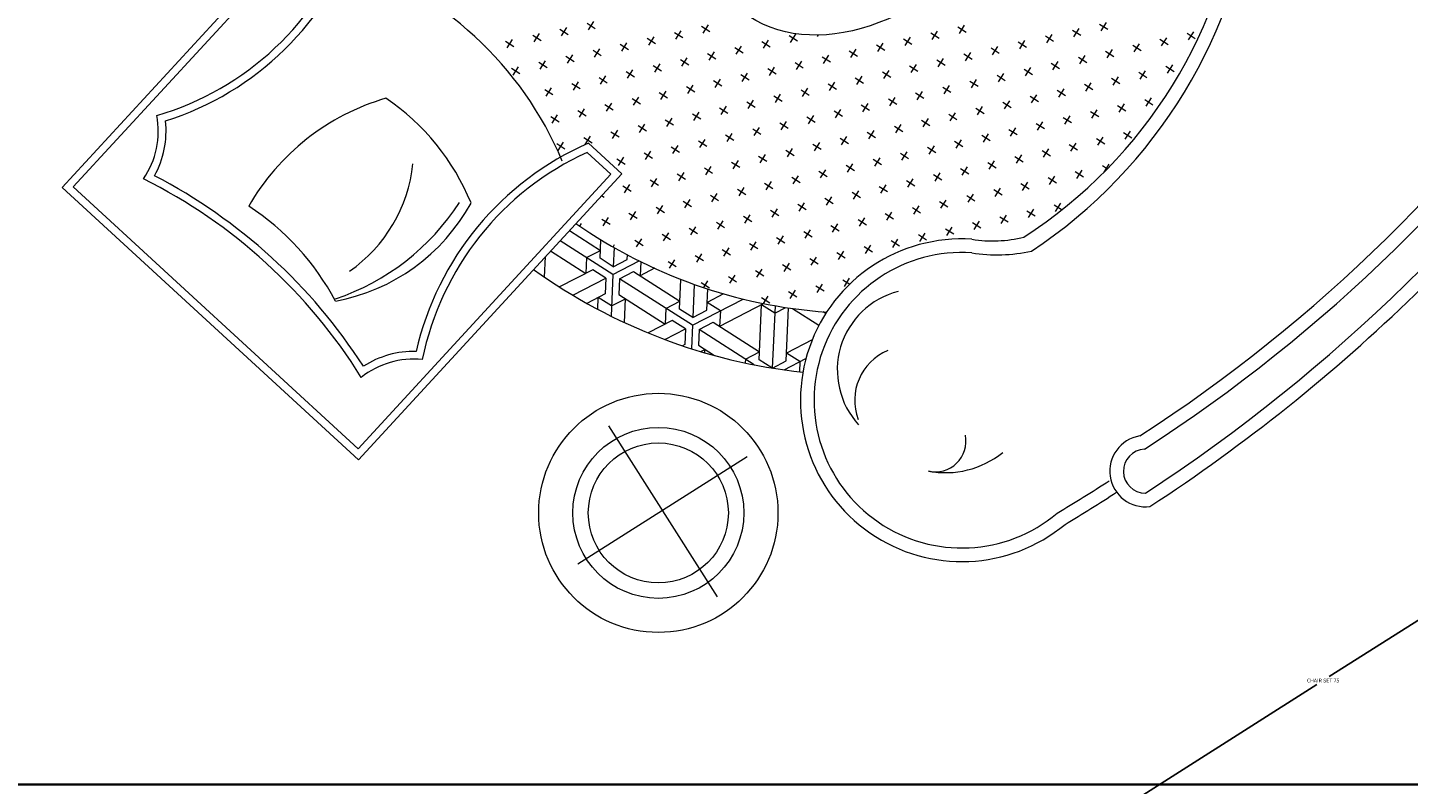
# Model space of a CAD drawing. Units: inches. Extents: x -4843 to -3402, y -164 to 3629.
# Tile 10 of 22: x -4532 to -4467, y 828 to 864. Entities that reach past the tile are written whole.
import ezdxf

# ---------------------------------------------------------------- set-up
doc = ezdxf.new("R2010")
doc.units = ezdxf.units.IN
for name, color, linetype, lineweight in [('A-ANNO-DIMS', 2, 'Continuous', 18), ('furniture', 6, 'Continuous', 18), ('walls', 7, 'Continuous', 35)]:
    doc.layers.add(name, color=color, linetype=linetype, lineweight=lineweight)
doc.styles.get("Standard").update_dxf_attribs({"font": 'arial.ttf'})
doc.dimstyles.get("Standard").update_dxf_attribs({"dimtxt": 0.18, "dimasz": 0.18, "dimexe": 0.18, "dimexo": 0.0625, "dimgap": 0.09, "dimtad": 0, "dimtih": 1, "dimtoh": 1, "dimdec": 4, "dimzin": 0, "dimdsep": 46, "dimtxsty": 'Standard', "dimcen": 0.09, "dimadec": 0, "dimazin": 0, "dimtfac": 1, "dimtdec": 4, "dimtofl": 0, "dimtmove": 0, "dimatfit": 3, "dimfxl": 1, "dimtolj": 1, "dimtzin": 0, "dimarcsym": 0})

# ---------------------------------------------------------------- blocks, each defined once
blk = doc.blocks.new('A$C30AE1D3B')
for p, q in [((2417.8, 2221.8, -685.7), (2417.8, 1828.4, -685.7)), ((2611.9, 2022.7, -685.7), (2223.7, 2022.7, -685.7)), ((1343.9, 1928.3, -685.7), (1327.1, 1920.4, -685.7)), ((1464.1, 1942.3, -685.7), (1446.8, 1934.2, -685.7)), ((1459.4, 1929.6, -685.7), (1451.7, 1946.1, -685.7)), ((1510.1, 1911.2, -685.7), (1502, 1928.4, -685.7)), ((2038.5, 1922.1, -685.7), (2049.7, 1938.2, -685.7)), ((1270.7, 1883.6, -685.7), (1262.6, 1900.9, -685.7)), ((1339.8, 1915.8, -685.7), (1334.9, 1926.2, -685.7)), ((1395, 1910.1, -685.7), (1377.7, 1902, -685.7)), ((1390.4, 1897.4, -685.7), (1382.3, 1914.7, -685.7)), ((1514.7, 1923.8, -685.7), (1497.4, 1915.8, -685.7)), ((1565.3, 1905.4, -685.7), (1548.1, 1897.3, -685.7)), ((1560.7, 1892.7, -685.7), (1552.7, 1910, -685.7)), ((2060.1, 1907, -685.7), (2001, 1822.6, -685.7)), ((2020.9, 1804.9, -685.7), (2090.2, 1904, -685.7)), ((2072.8, 1919.1, -685.7), (2025.3, 1923.3, -685.7)), ((2038.5, 1922.1, -685.7), (2051.4, 1894.5, -685.7)), ((2089.7, 1904.4, -685.7), (2060.1, 1907, -685.7)), ((2091, 1903.3, -685.7), (2103.3, 1876.7, -685.7)), ((1275.3, 1896.3, -685.7), (1258, 1888.2, -685.7)), ((1325.9, 1877.8, -685.7), (1308.7, 1869.8, -685.7)), ((1321.3, 1865.2, -685.7), (1313.3, 1882.5, -685.7)), ((1445.6, 1891.6, -685.7), (1428.4, 1883.6, -685.7)), ((1441, 1879, -685.7), (1433, 1896.2, -685.7)), ((1491.7, 1860.5, -685.7), (1483.6, 1877.8, -685.7)), ((1616, 1887, -685.7), (1598.7, 1878.9, -685.7)), ((1611.3, 1874.3, -685.7), (1603.3, 1891.6, -685.7)), ((1995.2, 1827.5, -685.7), (1969.6, 1882.5, -685.7)), ((1995.9, 1899.4, -685.7), (2051.4, 1894.5, -685.7)), ((2103.4, 1876.7, -685.7), (2042.2, 1789.3, -685.7)), ((2116.4, 1879.9, -685.7), (2170.1, 1764.9, -685.7)), ((1206.2, 1864.1, -685.7), (1189, 1856, -685.7)), ((1201.6, 1851.4, -685.7), (1193.6, 1868.7, -685.7)), ((1252.3, 1833, -685.7), (1244.2, 1850.3, -685.7)), ((1376.6, 1859.4, -685.7), (1359.3, 1851.4, -685.7)), ((1372, 1846.8, -685.7), (1363.9, 1864, -685.7)), ((1496.3, 1873.2, -685.7), (1479, 1865.1, -685.7)), ((1546.9, 1854.8, -685.7), (1529.6, 1846.7, -685.7)), ((1542.3, 1842.1, -685.7), (1534.2, 1859.4, -685.7)), ((1666.6, 1868.5, -685.7), (1649.3, 1860.5, -685.7)), ((1662, 1855.9, -685.7), (1653.9, 1873.1, -685.7)), ((1717.2, 1850.1, -685.7), (1700, 1842.1, -685.7)), ((1712.6, 1837.5, -685.7), (1704.6, 1854.7, -685.7)), ((1882.9, 1832.8, -685.7), (1876.2, 1847.2, -685.7)), ((1946.2, 1870.3, -685.7), (1948.8, 1864.7, -685.7)), ((2139.7, 1767.6, -685.7), (2094.6, 1864.2, -685.7)), ((2125, 1861.6, -685.7), (2094.6, 1864.2, -685.7)), ((2125, 1861.6, -685.7), (2129.2, 1867.6, -685.7)), ((1137.2, 1831.9, -685.7), (1119.9, 1823.8, -685.7)), ((1132.6, 1819.2, -685.7), (1124.5, 1836.5, -685.7)), ((1256.9, 1845.6, -685.7), (1239.6, 1837.6, -685.7)), ((1307.5, 1827.2, -685.7), (1290.2, 1819.2, -685.7)), ((1302.9, 1814.6, -685.7), (1294.8, 1831.8, -685.7)), ((1427.2, 1841, -685.7), (1409.9, 1832.9, -685.7)), ((1422.6, 1828.3, -685.7), (1414.5, 1845.6, -685.7)), ((1477.8, 1822.6, -685.7), (1460.6, 1814.5, -685.7)), ((1473.2, 1809.9, -685.7), (1465.2, 1827.2, -685.7)), ((1597.5, 1836.3, -685.7), (1580.3, 1828.3, -685.7)), ((1592.9, 1823.7, -685.7), (1584.9, 1840.9, -685.7)), ((1643.5, 1805.3, -685.7), (1635.5, 1822.5, -685.7)), ((1767.8, 1831.7, -685.7), (1750.6, 1823.6, -685.7)), ((1763.2, 1819, -685.7), (1755.2, 1836.3, -685.7)), ((1887.5, 1845.5, -685.7), (1870.3, 1837.4, -685.7)), ((1938.2, 1827, -685.7), (1920.9, 1819, -685.7)), ((1933.6, 1814.4, -685.7), (1925.5, 1831.6, -685.7)), ((2187.5, 1789.9, -685.7), (2172, 1823.3, -685.7)), ((1068.1, 1799.7, -685.7), (1050.9, 1791.6, -685.7)), ((1063.5, 1787, -685.7), (1055.5, 1804.3, -685.7)), ((1187.8, 1813.4, -685.7), (1170.5, 1805.4, -685.7)), ((1183.2, 1800.8, -685.7), (1175.2, 1818, -685.7)), ((1238.4, 1795, -685.7), (1221.2, 1787, -685.7)), ((1233.8, 1782.4, -685.7), (1225.8, 1799.6, -685.7)), ((1358.1, 1808.8, -685.7), (1340.9, 1800.7, -685.7)), ((1353.5, 1796.1, -685.7), (1345.5, 1813.4, -685.7)), ((1404.2, 1777.7, -685.7), (1396.1, 1795, -685.7)), ((1528.5, 1804.1, -685.7), (1511.2, 1796.1, -685.7)), ((1523.9, 1791.5, -685.7), (1515.8, 1808.7, -685.7)), ((1648.2, 1817.9, -685.7), (1630.9, 1809.9, -685.7)), ((1698.8, 1799.5, -685.7), (1681.5, 1791.4, -685.7)), ((1694.2, 1786.8, -685.7), (1686.1, 1804.1, -685.7)), ((1818.5, 1813.3, -685.7), (1801.2, 1805.2, -685.7)), ((1813.9, 1800.6, -685.7), (1805.8, 1817.9, -685.7)), ((1869.1, 1794.8, -685.7), (1851.8, 1786.8, -685.7)), ((1864.5, 1782.2, -685.7), (1856.5, 1799.4, -685.7)), ((1988.8, 1808.6, -685.7), (1971.5, 1800.6, -685.7)), ((1984.2, 1795.9, -685.7), (1976.1, 1813.2, -685.7)), ((2029.3, 1816.9, -685.7), (2005, 1819.1, -685.7)), ((2034.8, 1777.5, -685.7), (2026.8, 1794.8, -685.7)), ((2029.3, 1817, -685.7), (2042.2, 1789.3, -685.7)), ((2184.8, 1808.9, -685.7), (2181.1, 1803.7, -685.7)), ((2190.1, 1802.9, -685.7), (2181.1, 1803.7, -685.7)), ((1118.8, 1781.2, -685.7), (1101.5, 1773.2, -685.7)), ((1114.1, 1768.6, -685.7), (1106.1, 1785.8, -685.7)), ((1164.8, 1750.2, -685.7), (1156.7, 1767.4, -685.7)), ((1289.1, 1776.6, -685.7), (1271.8, 1768.5, -685.7)), ((1284.5, 1763.9, -685.7), (1276.4, 1781.2, -685.7)), ((1408.8, 1790.4, -685.7), (1391.5, 1782.3, -685.7)), ((1459.4, 1771.9, -685.7), (1442.1, 1763.9, -685.7)), ((1454.8, 1759.3, -685.7), (1446.7, 1776.5, -685.7)), ((1579.1, 1785.7, -685.7), (1561.8, 1777.7, -685.7)), ((1574.5, 1773, -685.7), (1566.4, 1790.3, -685.7)), ((1629.7, 1767.3, -685.7), (1612.5, 1759.2, -685.7)), ((1625.1, 1754.6, -685.7), (1617.1, 1771.9, -685.7)), ((1749.4, 1781.1, -685.7), (1732.2, 1773, -685.7)), ((1744.8, 1768.4, -685.7), (1736.8, 1785.7, -685.7)), ((1795.4, 1750, -685.7), (1787.4, 1767.2, -685.7)), ((1919.7, 1776.4, -685.7), (1902.5, 1768.3, -685.7)), ((1915.1, 1763.7, -685.7), (1907.1, 1781, -685.7)), ((2037.6, 1789.3, -685.7), (2022.2, 1782.1, -685.7)), ((2037.1, 1789.8, -685.7), (2133.3, 1781.4, -685.7)), ((2115.8, 1756.4, -685.7), (2133.3, 1781.4, -685.7)), ((2170.1, 1764.9, -685.7), (2139.7, 1767.5, -685.7)), ((2170.1, 1764.9, -685.7), (2187.6, 1789.9, -685.7)), ((2176.5, 1751.1, -685.7), (2202.5, 1788.2, -685.7)), ((2191.7, 1749.8, -685.7), (2209.2, 1774.7, -685.7)), ((2209.2, 1774.7, -685.7), (2214, 1774.3, -685.7)), ((1169.4, 1762.8, -685.7), (1152.1, 1754.8, -685.7)), ((1220, 1744.4, -685.7), (1202.8, 1736.3, -685.7)), ((1215.4, 1731.7, -685.7), (1207.4, 1749, -685.7)), ((1339.7, 1758.2, -685.7), (1322.4, 1750.1, -685.7)), ((1335.1, 1745.5, -685.7), (1327.1, 1762.8, -685.7)), ((1390.3, 1739.7, -685.7), (1373.1, 1731.7, -685.7)), ((1385.7, 1727.1, -685.7), (1377.7, 1744.3, -685.7)), ((1510, 1753.5, -685.7), (1492.8, 1745.5, -685.7)), ((1505.4, 1740.8, -685.7), (1497.4, 1758.1, -685.7)), ((1556.1, 1722.4, -685.7), (1548, 1739.7, -685.7)), ((1680.4, 1748.8, -685.7), (1663.1, 1740.8, -685.7)), ((1675.8, 1736.2, -685.7), (1667.7, 1753.5, -685.7)), ((1800.1, 1762.6, -685.7), (1782.8, 1754.6, -685.7)), ((1850.7, 1744.2, -685.7), (1833.4, 1736.1, -685.7)), ((1846.1, 1731.5, -685.7), (1838, 1748.8, -685.7)), ((1970.4, 1758, -685.7), (1953.1, 1749.9, -685.7)), ((1965.8, 1745.3, -685.7), (1957.7, 1762.6, -685.7)), ((2016.4, 1726.9, -685.7), (2008.4, 1744.1, -685.7)), ((2176.5, 1751.1, -685.7), (2066.2, 1760.7, -685.7)), ((2137.4, 1741.3, -685.7), (2113.7, 1707.4, -685.7)), ((2115.8, 1756.4, -685.7), (2128.6, 1728.8, -685.7)), ((2167.8, 1738.6, -685.7), (2137.4, 1741.2, -685.7)), ((2176.5, 1751.1, -685.7), (2247.3, 1599.2, -685.7)), ((2191.7, 1749.8, -685.7), (2204.6, 1722.1, -685.7)), ((2236.2, 1745.8, -685.7), (2191.7, 1749.7, -685.7)), ((1270.6, 1726, -685.7), (1253.4, 1717.9, -685.7)), ((1266, 1713.3, -685.7), (1258, 1730.6, -685.7)), ((1441, 1721.3, -685.7), (1423.7, 1713.2, -685.7)), ((1436.4, 1708.6, -685.7), (1428.3, 1725.9, -685.7)), ((1560.7, 1735.1, -685.7), (1543.4, 1727, -685.7)), ((1611.3, 1716.6, -685.7), (1594, 1708.6, -685.7)), ((1606.7, 1704, -685.7), (1598.6, 1721.3, -685.7)), ((1731, 1730.4, -685.7), (1713.7, 1722.4, -685.7)), ((1726.4, 1717.8, -685.7), (1718.3, 1735, -685.7)), ((1777, 1699.3, -685.7), (1769, 1716.6, -685.7)), ((1901.3, 1725.8, -685.7), (1884.1, 1717.7, -685.7)), ((1896.7, 1713.1, -685.7), (1888.7, 1730.4, -685.7)), ((2021, 1739.5, -685.7), (2003.7, 1731.5, -685.7)), ((2071.6, 1721.1, -685.7), (2054.4, 1713.1, -685.7)), ((2067, 1708.5, -685.7), (2059, 1725.7, -685.7)), ((2092.7, 1731.9, -685.7), (2128.7, 1728.8, -685.7)), ((2130.9, 1686, -685.7), (2167.8, 1738.6, -685.7)), ((2167.8, 1738.6, -685.7), (2180.6, 1711, -685.7)), ((2202.3, 1695.8, -685.7), (2219.8, 1720.8, -685.7)), ((2204.6, 1722.1, -685.7), (2256.9, 1717.5, -685.7)), ((2264.8, 1624.1, -685.7), (2219.7, 1720.8, -685.7)), ((1201.6, 1693.7, -685.7), (1184.3, 1685.7, -685.7)), ((1197, 1681.1, -685.7), (1188.9, 1698.4, -685.7)), ((1321.3, 1707.5, -685.7), (1304, 1699.5, -685.7)), ((1316.7, 1694.9, -685.7), (1308.6, 1712.1, -685.7)), ((1371.9, 1689.1, -685.7), (1354.6, 1681, -685.7)), ((1367.3, 1676.4, -685.7), (1359.3, 1693.7, -685.7)), ((1491.6, 1702.9, -685.7), (1474.3, 1694.8, -685.7)), ((1487, 1690.2, -685.7), (1478.9, 1707.5, -685.7)), ((1537.6, 1671.8, -685.7), (1529.6, 1689, -685.7)), ((1661.9, 1698.2, -685.7), (1644.7, 1690.2, -685.7)), ((1657.3, 1685.6, -685.7), (1649.3, 1702.8, -685.7)), ((1781.6, 1712, -685.7), (1764.4, 1703.9, -685.7)), ((1832.3, 1693.6, -685.7), (1815, 1685.5, -685.7)), ((1827.6, 1680.9, -685.7), (1819.6, 1698.2, -685.7)), ((1951.9, 1707.3, -685.7), (1934.7, 1699.3, -685.7)), ((1947.3, 1694.7, -685.7), (1939.3, 1711.9, -685.7)), ((2002.6, 1688.9, -685.7), (1985.3, 1680.9, -685.7)), ((1998, 1676.3, -685.7), (1989.9, 1693.5, -685.7)), ((2118.9, 1701.1, -685.7), (2105, 1694.6, -685.7)), ((2117.7, 1690, -685.7), (2109.6, 1707.3, -685.7)), ((2180.7, 1711, -685.7), (2147.7, 1663.9, -685.7)), ((2217, 1601.8, -685.7), (2171.9, 1698.5, -685.7)), ((2202.3, 1695.8, -685.7), (2171.9, 1698.5, -685.7)), ((1252.2, 1675.3, -685.7), (1235, 1667.3, -685.7)), ((1247.6, 1662.7, -685.7), (1239.6, 1679.9, -685.7)), ((1298.2, 1644.2, -685.7), (1290.2, 1661.5, -685.7)), ((1422.5, 1670.7, -685.7), (1405.3, 1662.6, -685.7)), ((1417.9, 1658, -685.7), (1409.9, 1675.3, -685.7)), ((1542.2, 1684.4, -685.7), (1525, 1676.4, -685.7)), ((1592.9, 1666, -685.7), (1575.6, 1658, -685.7)), ((1588.3, 1653.4, -685.7), (1580.2, 1670.6, -685.7)), ((1712.6, 1679.8, -685.7), (1695.3, 1671.7, -685.7)), ((1708, 1667.1, -685.7), (1699.9, 1684.4, -685.7)), ((1763.2, 1661.4, -685.7), (1745.9, 1653.3, -685.7)), ((1758.6, 1648.7, -685.7), (1750.5, 1666, -685.7)), ((1882.9, 1675.1, -685.7), (1865.6, 1667.1, -685.7)), ((1878.3, 1662.5, -685.7), (1870.2, 1679.7, -685.7)), ((1928.9, 1644, -685.7), (1920.9, 1661.3, -685.7)), ((2053.2, 1670.5, -685.7), (2035.9, 1662.4, -685.7)), ((2048.6, 1657.8, -685.7), (2040.6, 1675.1, -685.7)), ((2284.9, 1675.8, -685.7), (2258.4, 1637.9, -685.7)), ((1302.9, 1656.9, -685.7), (1285.6, 1648.8, -685.7)), ((1353.5, 1638.5, -685.7), (1336.2, 1630.4, -685.7)), ((1348.9, 1625.8, -685.7), (1340.8, 1643.1, -685.7)), ((1473.2, 1652.2, -685.7), (1455.9, 1644.2, -685.7)), ((1468.6, 1639.6, -685.7), (1460.5, 1656.8, -685.7)), ((1523.8, 1633.8, -685.7), (1506.5, 1625.8, -685.7)), ((1519.2, 1621.2, -685.7), (1511.2, 1638.4, -685.7)), ((1643.5, 1647.6, -685.7), (1626.2, 1639.5, -685.7)), ((1638.9, 1634.9, -685.7), (1630.8, 1652.2, -685.7)), ((1689.5, 1616.5, -685.7), (1681.5, 1633.8, -685.7)), ((1813.8, 1642.9, -685.7), (1796.6, 1634.9, -685.7)), ((1809.2, 1630.3, -685.7), (1801.2, 1647.5, -685.7)), ((1933.5, 1656.7, -685.7), (1916.3, 1648.7, -685.7)), ((1984.2, 1638.3, -685.7), (1966.9, 1630.2, -685.7)), ((1979.5, 1625.6, -685.7), (1971.5, 1642.9, -685.7)), ((2103.8, 1652.1, -685.7), (2086.6, 1644, -685.7)), ((2099.2, 1639.4, -685.7), (2091.2, 1656.7, -685.7)), ((2154.5, 1633.6, -685.7), (2137.2, 1625.6, -685.7)), ((2149.9, 1621, -685.7), (2141.8, 1638.2, -685.7)), ((2253.8, 1585.3, -685.7), (2300.1, 1651.4, -685.7)), ((2288.8, 1635.3, -685.7), (2258.4, 1637.9, -685.7)), ((2288.7, 1635.3, -685.7), (2301.6, 1607.7, -685.7)), ((1404.1, 1620, -685.7), (1386.9, 1612, -685.7)), ((1399.5, 1607.4, -685.7), (1391.5, 1624.6, -685.7)), ((1450.1, 1588.9, -685.7), (1442.1, 1606.2, -685.7)), ((1574.4, 1615.4, -685.7), (1557.2, 1607.3, -685.7)), ((1569.8, 1602.7, -685.7), (1561.8, 1620, -685.7)), ((1694.1, 1629.2, -685.7), (1676.9, 1621.1, -685.7)), ((1744.8, 1610.7, -685.7), (1727.5, 1602.7, -685.7)), ((1740.2, 1598.1, -685.7), (1732.1, 1615.3, -685.7)), ((1864.5, 1624.5, -685.7), (1847.2, 1616.5, -685.7)), ((1859.9, 1611.8, -685.7), (1851.8, 1629.1, -685.7)), ((1915.1, 1606.1, -685.7), (1897.8, 1598, -685.7)), ((1910.5, 1593.4, -685.7), (1902.4, 1610.7, -685.7)), ((2034.8, 1619.8, -685.7), (2017.5, 1611.8, -685.7)), ((2030.2, 1607.2, -685.7), (2022.1, 1624.5, -685.7)), ((2080.8, 1588.8, -685.7), (2072.8, 1606, -685.7)), ((2134.6, 1429.4, -685.7), (2862.6, 1623.9, -685.7)), ((2179.2, 1618.3, -685.7), (2210.5, 1615.6, -685.7)), ((2195, 1593.3, -685.7), (2210.6, 1615.6, -685.7)), ((2247.4, 1599.2, -685.7), (2264.8, 1624.1, -685.7)), ((2269, 1584, -685.7), (2286.5, 1609, -685.7)), ((2286.5, 1609, -685.7), (2326.2, 1605.5, -685.7)), ((2314.7, 1626.3, -685.7), (2301.7, 1607.7, -685.7)), ((2862.6, 1623.9, -685.7), (3064, 870.4, -685.7)), ((1454.7, 1601.6, -685.7), (1437.5, 1593.6, -685.7)), ((1505.4, 1583.2, -685.7), (1488.1, 1575.1, -685.7)), ((1500.8, 1570.5, -685.7), (1492.7, 1587.8, -685.7)), ((1625.1, 1597, -685.7), (1607.8, 1588.9, -685.7)), ((1620.5, 1584.3, -685.7), (1612.4, 1601.6, -685.7)), ((1671.1, 1565.9, -685.7), (1663, 1583.1, -685.7)), ((1795.4, 1592.3, -685.7), (1778.1, 1584.2, -685.7)), ((1790.8, 1579.6, -685.7), (1782.7, 1596.9, -685.7)), ((1965.7, 1587.6, -685.7), (1948.5, 1579.6, -685.7)), ((1961.1, 1575, -685.7), (1953.1, 1592.3, -685.7)), ((2085.4, 1601.4, -685.7), (2068.2, 1593.4, -685.7)), ((2136, 1583, -685.7), (2118.8, 1574.9, -685.7)), ((2131.4, 1570.3, -685.7), (2123.4, 1587.6, -685.7)), ((2152.9, 1418.8, -685.7), (2852, 1605.6, -685.7)), ((2253.8, 1585.3, -685.7), (2196.8, 1590.3, -685.7)), ((2247.3, 1599.1, -685.7), (2217, 1601.8, -685.7)), ((2253.8, 1585.3, -685.7), (2305.2, 1475, -685.7)), ((2269, 1584, -685.7), (2281.8, 1556.4, -685.7)), ((2340.7, 1577.7, -685.7), (2269, 1584, -685.7)), ((2852, 1605.6, -685.7), (3045.6, 881, -685.7)), ((1431.7, 1538.3, -685.7), (1423.7, 1555.6, -685.7)), ((1556, 1564.7, -685.7), (1538.7, 1556.7, -685.7)), ((1551.4, 1552.1, -685.7), (1543.4, 1569.4, -685.7)), ((1675.7, 1578.5, -685.7), (1658.4, 1570.5, -685.7)), ((1726.3, 1560.1, -685.7), (1709.1, 1552, -685.7)), ((1721.7, 1547.4, -685.7), (1713.7, 1564.7, -685.7)), ((1846, 1573.9, -685.7), (1828.8, 1565.8, -685.7)), ((1841.4, 1561.2, -685.7), (1833.4, 1578.5, -685.7)), ((1896.7, 1555.4, -685.7), (1879.4, 1547.4, -685.7)), ((1892.1, 1542.8, -685.7), (1884, 1560, -685.7)), ((2016.4, 1569.2, -685.7), (1999.1, 1561.2, -685.7)), ((2011.7, 1556.6, -685.7), (2003.7, 1573.8, -685.7)), ((2062.4, 1538.1, -685.7), (2054.3, 1555.4, -685.7)), ((2186.7, 1564.6, -685.7), (2169.4, 1556.5, -685.7)), ((2182.1, 1551.9, -685.7), (2174, 1569.2, -685.7)), ((2214.7, 1575.5, -685.7), (2209.7, 1568.3, -685.7)), ((2245, 1572.8, -685.7), (2214.7, 1575.5, -685.7)), ((2223.8, 1542.5, -685.7), (2245.1, 1572.9, -685.7)), ((2245, 1572.9, -685.7), (2257.9, 1545.2, -685.7)), ((2279.6, 1530.1, -685.7), (2297, 1555.1, -685.7)), ((2281.9, 1556.4, -685.7), (2354.1, 1550.1, -685.7)), ((2331.1, 1481.9, -685.7), (2297, 1555.1, -685.7)), ((1436.3, 1551, -685.7), (1419.1, 1542.9, -685.7)), ((1487, 1532.5, -685.7), (1469.7, 1524.5, -685.7)), ((1482.3, 1519.9, -685.7), (1474.3, 1537.2, -685.7)), ((1606.6, 1546.3, -685.7), (1589.4, 1538.3, -685.7)), ((1602, 1533.7, -685.7), (1594, 1550.9, -685.7)), ((1657.3, 1527.9, -685.7), (1640, 1519.8, -685.7)), ((1652.7, 1515.2, -685.7), (1644.6, 1532.5, -685.7)), ((1777, 1541.7, -685.7), (1759.7, 1533.6, -685.7)), ((1772.4, 1529, -685.7), (1764.3, 1546.3, -685.7)), ((1823, 1510.6, -685.7), (1814.9, 1527.8, -685.7)), ((1947.3, 1537, -685.7), (1930, 1529, -685.7)), ((1942.7, 1524.4, -685.7), (1934.6, 1541.6, -685.7)), ((2067, 1550.8, -685.7), (2049.7, 1542.7, -685.7)), ((2117.6, 1532.4, -685.7), (2100.4, 1524.3, -685.7)), ((2113, 1519.7, -685.7), (2105, 1537, -685.7)), ((2225, 1540.4, -685.7), (2220, 1538.1, -685.7)), ((2257.9, 1545.2, -685.7), (2237.4, 1515.9, -685.7)), ((2279.3, 1468.1, -685.7), (2249.2, 1532.8, -685.7)), ((2279.6, 1530.1, -685.7), (2249.2, 1532.7, -685.7)), ((1537.6, 1514.1, -685.7), (1520.3, 1506.1, -685.7)), ((1533, 1501.5, -685.7), (1524.9, 1518.7, -685.7)), ((1583.6, 1483, -685.7), (1575.6, 1500.3, -685.7)), ((1707.9, 1509.5, -685.7), (1690.6, 1501.4, -685.7)), ((1703.3, 1496.8, -685.7), (1695.3, 1514.1, -685.7)), ((1827.6, 1523.2, -685.7), (1810.3, 1515.2, -685.7)), ((1878.2, 1504.8, -685.7), (1861, 1496.8, -685.7)), ((1873.6, 1492.2, -685.7), (1865.6, 1509.4, -685.7)), ((1997.9, 1518.6, -685.7), (1980.7, 1510.5, -685.7)), ((1993.3, 1505.9, -685.7), (1985.3, 1523.2, -685.7)), ((2048.6, 1500.2, -685.7), (2031.3, 1492.1, -685.7)), ((2044, 1487.5, -685.7), (2035.9, 1504.8, -685.7)), ((2168.3, 1513.9, -685.7), (2151, 1505.9, -685.7)), ((2163.6, 1501.3, -685.7), (2155.6, 1518.5, -685.7)), ((2214.3, 1482.8, -685.7), (2206.2, 1500.1, -685.7)), ((2368.2, 1518.5, -685.7), (2345.1, 1485.7, -685.7)), ((1588.2, 1495.7, -685.7), (1571, 1487.6, -685.7)), ((1638.8, 1477.3, -685.7), (1621.6, 1469.2, -685.7)), ((1634.2, 1464.6, -685.7), (1626.2, 1481.9, -685.7)), ((1758.5, 1491, -685.7), (1741.3, 1483, -685.7)), ((1753.9, 1478.4, -685.7), (1745.9, 1495.6, -685.7)), ((1809.2, 1472.6, -685.7), (1791.9, 1464.6, -685.7)), ((1804.6, 1459.9, -685.7), (1796.5, 1477.2, -685.7)), ((1928.9, 1486.4, -685.7), (1911.6, 1478.3, -685.7)), ((1924.3, 1473.7, -685.7), (1916.2, 1491, -685.7)), ((1974.9, 1455.3, -685.7), (1966.8, 1472.6, -685.7)), ((2099.2, 1481.7, -685.7), (2081.9, 1473.7, -685.7)), ((2094.6, 1469.1, -685.7), (2086.5, 1486.3, -685.7)), ((2218.9, 1495.5, -685.7), (2201.6, 1487.5, -685.7)), ((1689.5, 1458.8, -685.7), (1672.2, 1450.8, -685.7)), ((1684.9, 1446.2, -685.7), (1676.8, 1463.4, -685.7)), ((1859.8, 1454.2, -685.7), (1842.5, 1446.1, -685.7)), ((1855.2, 1441.5, -685.7), (1847.1, 1458.8, -685.7)), ((1979.5, 1468, -685.7), (1962.2, 1459.9, -685.7)), ((2030.1, 1449.5, -685.7), (2012.9, 1441.5, -685.7)), ((2025.5, 1436.9, -685.7), (2017.5, 1454.1, -685.7)), ((2149.8, 1463.3, -685.7), (2132.6, 1455.2, -685.7)), ((2145.2, 1450.6, -685.7), (2137.2, 1467.9, -685.7)), ((2190.2, 1444.3, -685.7), (2187.8, 1449.5, -685.7)), ((2257.7, 1471.6, -685.7), (2252.2, 1469, -685.7)), ((1740.1, 1440.4, -685.7), (1722.8, 1432.4, -685.7)), ((1735.5, 1427.7, -685.7), (1727.5, 1445, -685.7)), ((1790.7, 1422, -685.7), (1773.5, 1413.9, -685.7)), ((1786.1, 1409.3, -685.7), (1778.1, 1426.6, -685.7)), ((1910.4, 1435.7, -685.7), (1893.2, 1427.7, -685.7)), ((1905.8, 1423.1, -685.7), (1897.8, 1440.4, -685.7)), ((1956.5, 1404.7, -685.7), (1948.4, 1421.9, -685.7)), ((2080.8, 1431.1, -685.7), (2063.5, 1423, -685.7)), ((2076.2, 1418.4, -685.7), (2068.1, 1435.7, -685.7)), ((2157.1, 1345, -685.7), (2134.6, 1429.4, -685.7)), ((2169.1, 1358.4, -685.7), (2152.9, 1418.8, -685.7)), ((1658.5, 1412.5, -685.7), (1658.4, 1412.8, -685.7)), ((1671.1, 1408.2, -685.7), (1668.2, 1406.9, -685.7)), ((1717.1, 1377.1, -685.7), (1709, 1394.4, -685.7)), ((1841.4, 1403.5, -685.7), (1824.1, 1395.5, -685.7)), ((1836.8, 1390.9, -685.7), (1828.7, 1408.2, -685.7)), ((1961.1, 1417.3, -685.7), (1943.8, 1409.3, -685.7)), ((2011.7, 1398.9, -685.7), (1994.4, 1390.8, -685.7)), ((2007.1, 1386.2, -685.7), (1999, 1403.5, -685.7)), ((2131.4, 1412.7, -685.7), (2114.1, 1404.6, -685.7)), ((2126.8, 1400, -685.7), (2118.7, 1417.3, -685.7)), ((1721.7, 1389.8, -685.7), (1704.4, 1381.7, -685.7)), ((1772.3, 1371.3, -685.7), (1755.1, 1363.3, -685.7)), ((1767.7, 1358.7, -685.7), (1759.7, 1375.9, -685.7)), ((1892, 1385.1, -685.7), (1874.7, 1377.1, -685.7)), ((1887.4, 1372.5, -685.7), (1879.4, 1389.7, -685.7)), ((1942.6, 1366.7, -685.7), (1925.4, 1358.6, -685.7)), ((1938, 1354, -685.7), (1930, 1371.3, -685.7)), ((2062.3, 1380.5, -685.7), (2045.1, 1372.4, -685.7)), ((2057.7, 1367.8, -685.7), (2049.7, 1385.1, -685.7)), ((2108.4, 1349.4, -685.7), (2100.3, 1366.6, -685.7)), ((1822.9, 1352.9, -685.7), (1805.7, 1344.9, -685.7)), ((1818.3, 1340.3, -685.7), (1810.3, 1357.5, -685.7)), ((1869, 1321.8, -685.7), (1860.9, 1339.1, -685.7)), ((1993.3, 1348.3, -685.7), (1976, 1340.2, -685.7)), ((1988.7, 1335.6, -685.7), (1980.6, 1352.9, -685.7)), ((2113, 1362, -685.7), (2095.7, 1354, -685.7)), ((2163.6, 1343.6, -685.7), (2146.3, 1335.6, -685.7)), ((2159, 1330.9, -685.7), (2150.9, 1348.2, -685.7)), ((1873.6, 1334.5, -685.7), (1856.3, 1326.4, -685.7)), ((1924.2, 1316.1, -685.7), (1906.9, 1308, -685.7)), ((1919.6, 1303.4, -685.7), (1911.6, 1320.7, -685.7)), ((2043.9, 1329.8, -685.7), (2026.6, 1321.8, -685.7)), ((2039.3, 1317.2, -685.7), (2031.2, 1334.4, -685.7)), ((2089.9, 1298.7, -685.7), (2081.9, 1316, -685.7)), ((2214.2, 1325.2, -685.7), (2197, 1317.1, -685.7)), ((2209.6, 1312.5, -685.7), (2201.6, 1329.8, -685.7)), ((1850.5, 1271.2, -685.7), (1842.5, 1288.5, -685.7)), ((1974.8, 1297.6, -685.7), (1957.6, 1289.6, -685.7)), ((1970.2, 1285, -685.7), (1962.2, 1302.2, -685.7)), ((2094.5, 1311.4, -685.7), (2077.3, 1303.4, -685.7)), ((2145.2, 1293, -685.7), (2127.9, 1284.9, -685.7)), ((2140.6, 1280.3, -685.7), (2132.5, 1297.6, -685.7)), ((1855.2, 1283.9, -685.7), (1837.9, 1275.8, -685.7)), ((1905.8, 1265.4, -685.7), (1888.5, 1257.4, -685.7)), ((1901.2, 1252.8, -685.7), (1893.1, 1270, -685.7)), ((2025.5, 1279.2, -685.7), (2008.2, 1271.1, -685.7)), ((2020.9, 1266.5, -685.7), (2012.8, 1283.8, -685.7)), ((2076.1, 1260.8, -685.7), (2058.8, 1252.7, -685.7)), ((2071.5, 1248.1, -685.7), (2063.4, 1265.4, -685.7)), ((2195.8, 1274.5, -685.7), (2178.5, 1266.5, -685.7)), ((2191.2, 1261.9, -685.7), (2183.1, 1279.2, -685.7)), ((1956.4, 1247, -685.7), (1939.2, 1238.9, -685.7)), ((1951.8, 1234.3, -685.7), (1943.8, 1251.6, -685.7)), ((2002.4, 1215.9, -685.7), (1994.4, 1233.2, -685.7)), ((2126.7, 1242.3, -685.7), (2109.5, 1234.3, -685.7)), ((2122.1, 1229.7, -685.7), (2114.1, 1246.9, -685.7)), ((2007, 1228.6, -685.7), (1989.8, 1220.5, -685.7)), ((2057.7, 1210.1, -685.7), (2040.4, 1202.1, -685.7)), ((2053.1, 1197.5, -685.7), (2045, 1214.7, -685.7)), ((2177.4, 1223.9, -685.7), (2160.1, 1215.9, -685.7)), ((2172.8, 1211.3, -685.7), (2164.7, 1228.5, -685.7)), ((2108.3, 1191.7, -685.7), (2091, 1183.7, -685.7)), ((2103.7, 1179.1, -685.7), (2095.7, 1196.3, -685.7)), ((2154.3, 1160.6, -685.7), (2146.3, 1177.9, -685.7)), ((2039.3, 1159.5, -685.7), (2022, 1151.5, -685.7)), ((2034.6, 1146.8, -685.7), (2026.6, 1164.1, -685.7)), ((2158.9, 1173.3, -685.7), (2141.7, 1165.2, -685.7)), ((2209.6, 1154.9, -685.7), (2192.3, 1146.8, -685.7)), ((2205, 1142.2, -685.7), (2196.9, 1159.5, -685.7)), ((2089.9, 1141.1, -685.7), (2072.6, 1133, -685.7)), ((2085.3, 1128.4, -685.7), (2077.2, 1145.7, -685.7)), ((2135.9, 1110, -685.7), (2127.9, 1127.3, -685.7)), ((2140.5, 1122.6, -685.7), (2123.2, 1114.6, -685.7)), ((2191.1, 1104.2, -685.7), (2173.9, 1096.2, -685.7)), ((2186.5, 1091.6, -685.7), (2178.5, 1108.8, -685.7)), ((2225.7, 1078.3, -685.7), (2224.5, 1077.7, -685.7)), ((3064, 870.4, -685.7), (2336, 675.8, -685.7)), ((3045.6, 881, -685.7), (2346.6, 694.2, -685.7))]:
    blk.add_line(p, q)
for radius in [231.9, 165.7, 135.7]:
    blk.add_circle((2427.4, 2022.7, -685.7), radius)
for centre, radius, start, end in [((1659.5, -897.1, -685.7), 3420.6, 90.7208, 112.8056), ((1587.1, 2460.7, -685.7), 69.1, 246.7414, 64.8312), ((1659.5, -897.1, -685.7), 3394.2, 90.8361, 112.7864), ((1587.1, 2460.7, -685.7), 42.7, 240.1456, 57.5884), ((1813.7, 2153.8, -685.7), 312.9, 234.002, 97.2975), ((1685.5, -1256.8, -685.7), 3722.1, 88.6375, 90.4534), ((1813.7, 2153.8, -685.7), 286.5, 233.7284, 97.6892), ((1685.5, -1256.8, -685.7), 3695.7, 88.6059, 90.4534), ((1588.1, -668.8, -685.7), 3092.5, 90.4124, 113.4876), ((1588.1, -668.8, -685.7), 3066.1, 90.5286, 113.4647), ((1820.7, 2106.3, -685.7), 176.7, 46.6292, 96.2845), ((1899.6, 2193.7, -685.7), 59.1, 44.0502, 159.0618), ((1853.1, 2059.3, -685.7), 157.5, 252.0328, 10.0812), ((1901, 2098, -685.7), 104, 260.1804, 348.5783), ((1564.8, 996.8, -685.7), 985.5, 91.1759, 141.3181), ((1432.1, 1679.7, -685.7), 322.7, 48.8986, 69.5858), ((1550.3, 1015.2, -685.7), 936.1, 90.475, 141.314), ((1463.9, 1715.4, -685.7), 248.6, 48.16, 71.5623), ((1366.9, 1089.4, -685.7), 1089.4, 21.8308, 51.5393), ((1366.9, 1089.4, -685.7), 969.4, 22.686, 53.5264), ((2246.2, 1919.7, -685.7), 566.6, 262.1788, 316.0405), ((2755.4, 1654.6, -685.7), 163.4, 231.6723, 275.9888), ((2246.2, 1919.7, -685.7), 581.6, 261.1931, 314.7504), ((2755.4, 1654.6, -685.7), 178.4, 236.0104, 270.6505), ((3827.7, 1482.5, -685.7), 1070.3, 180.3382, 210.0194), ((3827.7, 1482.5, -685.7), 1055.3, 179.4809, 210.8948), ((2594.1, 990.5, -685.7), 377.3, 67.9806, 118.9326), ((2899.7, 1230.2, -685.7), 690.9, 170.2555, 219.6682), ((2622.8, 887.8, -685.7), 462.2, 76.23, 114.7049), ((3221, 1299.4, -685.7), 487.2, 175.186, 204.8059), ((2853.2, 1240.6, -685.7), 448.9, 169.725, 203.6172), ((2693.4, 1016.2, -685.7), 290.1, 92.3667, 141.6364), ((2567.9, 1495.9, -685.7), 453, 253.8506, 297.7344), ((2986.3, 790.4, -685.7), 178.4, 118.5861, 153.9133), ((2986.3, 790.4, -685.7), 163.4, 113.1358, 158.2514), ((2677.3, 306.6, -685.7), 581.6, 75.1733, 128.7306), ((2677.3, 306.6, -685.7), 566.6, 73.8832, 127.7449)]:
    blk.add_arc(centre, radius, start, end)
blk.add_ellipse((1353.7, 1139.3, -685.7), major_axis=(414.6, 150.9), ratio=0.680002)
blk = doc.blocks.new('*D50')
at = {"layer": 'A-ANNO-DIMS', "color": 0, "lineweight": -2, "transparency": 16777216}
for p, q in [((-4445.305, 862.819), (-4439.203, 853.213)), ((-4439.451, 853.269), (-4470.698, 833.416)), ((-4502.521, 813.197), (-4471.274, 833.05)), ((-4508.679, 822.554), (-4502.577, 812.949))]:
    blk.add_line(p, q, dxfattribs=at)
at = {"layer": 'A-ANNO-DIMS', "color": 0, "transparency": 16777216}
for points in [[(-4439.467, 853.294), (-4439.435, 853.243), (-4439.299, 853.365)], [(-4502.537, 813.222), (-4502.505, 813.172), (-4502.673, 813.101)]]:
    blk.add_solid(points, dxfattribs=at)
at = {"layer": 'Defpoints', "color": 0, "transparency": 16777216}
for p in [(-4445.339, 862.871), (-4508.713, 822.607), (-4502.673, 813.101)]:
    blk.add_point(p, dxfattribs=at)
at = {"layer": 'A-ANNO-DIMS', "color": 0, "transparency": 16777216, "insert": (-4470.986, 833.233), "char_height": 0.18, "attachment_point": 5}
blk.add_mtext('\\A1;CHAIR SET 75', dxfattribs=at)
blk = doc.blocks.new('*D51')
at = {"layer": 'A-ANNO-DIMS', "color": 0, "lineweight": -2, "transparency": 16777216}
for p, q in [((-4479.57, 916.866), (-4469.965, 922.969)), ((-4470.021, 922.721), (-4453.091, 896.074)), ((-4435.929, 869.063), (-4452.859, 895.71)), ((-4445.286, 862.905), (-4435.681, 869.008))]:
    blk.add_line(p, q, dxfattribs=at)
at = {"layer": 'A-ANNO-DIMS', "color": 0, "transparency": 16777216}
for points in [[(-4469.995, 922.737), (-4470.046, 922.704), (-4470.117, 922.872)], [(-4435.904, 869.079), (-4435.955, 869.047), (-4435.833, 868.911)]]:
    blk.add_solid(points, dxfattribs=at)
at = {"layer": 'Defpoints', "color": 0, "transparency": 16777216}
for p in [(-4479.623, 916.833), (-4435.833, 868.911), (-4445.339, 862.871)]:
    blk.add_point(p, dxfattribs=at)
at = {"layer": 'A-ANNO-DIMS', "color": 0, "transparency": 16777216, "insert": (-4452.975, 895.892), "char_height": 0.18, "attachment_point": 5}
blk.add_mtext('\\A1;64', dxfattribs=at)

msp = doc.modelspace()

# ---------------------------------------------------------------- linework, layer by layer
at = {"layer": 'walls'}
msp.add_line((-4586.783, 828.354), (-4460.783, 828.354), dxfattribs=at)

# ---------------------------------------------------------------- block references
at = {"layer": 'furniture', "xscale": 0.0242257431082848, "yscale": 0.0242257431082848, "zscale": 0.0242257431082848, "rotation": 212.4298414976532}
msp.add_blockref('A$C30AE1D3B', (-4478.842, 914.005, -463.669), dxfattribs=at)

# ---------------------------------------------------------------- dimensions: what is measured, and where the dimension line sits
at = {"layer": 'A-ANNO-DIMS'}
dim = msp.add_linear_dim(base=(-4435.833, 868.911), p1=(-4479.623, 916.833), p2=(-4445.339, 862.871), angle=302.42984, dimstyle='Standard', override={"dimdec": 0, "dimlfac": 1, "dimrnd": 0, "dimzin": 0, "dimdsep": 46, "dimlunit": 2}, dxfattribs=at)
dim.commit()
dim.dimension.update_dxf_attribs({"geometry": '*D51', "text_midpoint": (-4452.975, 895.892)})
dim = msp.add_linear_dim(base=(-4502.673, 813.101), p1=(-4445.339, 862.871), p2=(-4508.713, 822.607), angle=212.42984, text='CHAIR SET <>', dimstyle='Standard', override={"dimdec": 0, "dimlfac": 1, "dimrnd": 0, "dimzin": 0, "dimdsep": 46, "dimlunit": 2}, dxfattribs=at)
dim.commit()
dim.dimension.update_dxf_attribs({"geometry": '*D50', "text_midpoint": (-4470.986, 833.233)})

doc.saveas('drawing.dxf')
